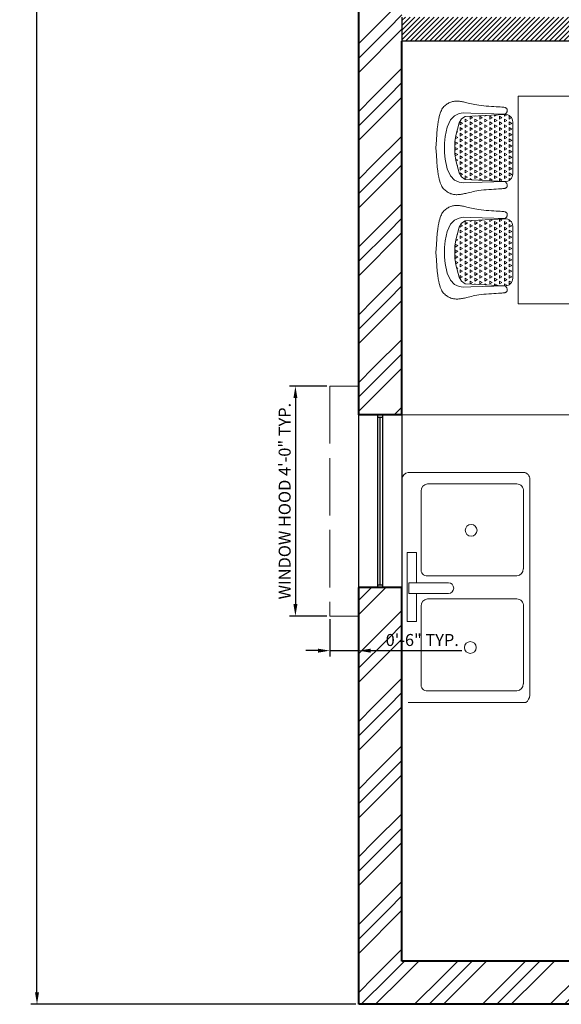
# Model space of a CAD drawing. Units: inches. Extents: x 2443635 to 2446153, y 1826255 to 1827341.
# Tile 6 of 16: x 2444253 to 2444366, y 1826861 to 1827067. Entities that reach past the tile are written whole.
import ezdxf

# ---------------------------------------------------------------- set-up
doc = ezdxf.new("R2010")
doc.units = ezdxf.units.IN
doc.linetypes.add('ACAD_ISO02W100', pattern=[15, 12, -3])
for name, color, linetype, lineweight in [('A-DIMS', 1, 'Continuous', 18), ('A-FLOR-CASE', 8, 'Continuous', 18), ('A-FLOR-FIXT', 9, 'Continuous', 18), ('A-FURN', 6, 'Continuous', 18), ('A-WALL-EXT', 7, 'Continuous', 40), ('A-WALL-INT', 9, 'Continuous', 30), ('A-WALL-OVHD', 7, 'ACAD_ISO02W100', 18), ('A-WALL-PATT', 8, 'Continuous', 13), ('A-WINDOW', 4, 'Continuous', 25)]:
    doc.layers.add(name, color=color, linetype=linetype, lineweight=lineweight)
doc.styles.get("Standard").update_dxf_attribs({"font": 'arial.ttf'})
doc.dimstyles.new('ISO-25', dxfattribs={"dimtxt": 2.5, "dimasz": 2.5, "dimexe": 1.25, "dimexo": 0.625, "dimtad": 1, "dimlunit": 4, "dimtxsty": 'Standard', "dimcen": 2.5, "dimadec": 0, "dimazin": 0, "dimtfac": 1, "dimtmove": 0, "dimatfit": 3, "dimfxl": 1, "dimarcsym": 0})

# ---------------------------------------------------------------- blocks, each defined once
blk = doc.blocks.new('*X10')
at = {"color": 0}
for p, q in [((152.44, 136.07), (152.22, 136.07)), ((152.35, 136.23), (152.44, 136.07)), ((152.62, 135.75), (152.44, 135.42)), ((152.62, 135.75), (152.81, 135.42)), ((153, 136.4), (152.81, 136.07)), ((153.19, 136.07), (152.81, 136.07)), ((153, 136.4), (153.19, 136.07)), ((153.37, 135.75), (153.19, 135.42)), ((153.37, 135.75), (153.56, 135.42)), ((153.75, 136.4), (153.56, 136.07)), ((153.94, 136.07), (153.56, 136.07)), ((153.75, 136.4), (153.94, 136.07)), ((154.12, 135.75), (153.94, 135.42)), ((154.12, 135.75), (154.31, 135.42)), ((154.5, 136.4), (154.31, 136.07)), ((154.69, 136.07), (154.31, 136.07)), ((154.5, 136.4), (154.69, 136.07)), ((154.87, 135.75), (154.69, 135.42)), ((154.87, 135.75), (155.06, 135.42)), ((155.25, 136.4), (155.06, 136.07)), ((155.44, 136.07), (155.06, 136.07)), ((155.25, 136.4), (155.44, 136.07)), ((155.62, 135.75), (155.44, 135.42)), ((155.62, 135.75), (155.81, 135.42)), ((156, 136.4), (155.81, 136.07)), ((156.19, 136.07), (155.81, 136.07)), ((156, 136.4), (156.19, 136.07)), ((156.37, 135.75), (156.19, 135.42)), ((156.37, 135.75), (156.56, 135.42)), ((156.75, 136.4), (156.56, 136.07)), ((156.94, 136.07), (156.56, 136.07)), ((156.75, 136.4), (156.94, 136.07)), ((157.12, 135.75), (156.94, 135.42)), ((157.12, 135.75), (157.31, 135.42)), ((157.5, 136.4), (157.31, 136.07)), ((157.69, 136.07), (157.31, 136.07)), ((157.5, 136.4), (157.69, 136.07)), ((157.87, 135.75), (157.69, 135.42)), ((157.87, 135.75), (158.06, 135.42)), ((158.25, 136.4), (158.06, 136.07)), ((158.44, 136.07), (158.06, 136.07)), ((158.25, 136.4), (158.44, 136.07)), ((158.62, 135.75), (158.44, 135.42)), ((158.62, 135.75), (158.81, 135.42)), ((159, 136.4), (158.81, 136.07)), ((159.19, 136.07), (158.81, 136.07)), ((159, 136.4), (159.19, 136.07)), ((159.37, 135.75), (159.19, 135.42)), ((159.37, 135.75), (159.56, 135.42)), ((159.75, 136.4), (159.56, 136.07)), ((159.94, 136.07), (159.56, 136.07)), ((159.75, 136.4), (159.94, 136.07)), ((160.12, 135.75), (159.94, 135.42)), ((160.12, 135.75), (160.31, 135.42)), ((160.48, 136.37), (160.31, 136.07)), ((160.69, 136.07), (160.31, 136.07)), ((160.54, 136.33), (160.69, 136.07)), ((160.87, 135.75), (160.69, 135.42)), ((160.87, 135.75), (160.94, 135.64)), ((152.06, 135.44), (152.06, 135.42)), ((152.06, 135.42), (152.06, 135.42)), ((152.25, 135.1), (152.09, 134.82)), ((152.44, 134.78), (152.09, 134.78)), ((152.25, 135.1), (152.44, 134.78)), ((152.81, 135.42), (152.44, 135.42)), ((152.62, 134.45), (152.44, 134.13)), ((152.62, 134.45), (152.81, 134.13)), ((153, 135.1), (152.81, 134.78)), ((153.19, 134.78), (152.81, 134.78)), ((153, 135.1), (153.19, 134.78)), ((153.56, 135.42), (153.19, 135.42)), ((153.37, 134.45), (153.19, 134.13)), ((153.37, 134.45), (153.56, 134.13)), ((153.75, 135.1), (153.56, 134.78)), ((153.94, 134.78), (153.56, 134.78)), ((153.75, 135.1), (153.94, 134.78)), ((154.31, 135.42), (153.94, 135.42)), ((154.12, 134.45), (153.94, 134.13)), ((154.12, 134.45), (154.31, 134.13)), ((154.5, 135.1), (154.31, 134.78)), ((154.69, 134.78), (154.31, 134.78)), ((154.5, 135.1), (154.69, 134.78)), ((155.06, 135.42), (154.69, 135.42)), ((154.87, 134.45), (154.69, 134.13)), ((154.87, 134.45), (155.06, 134.13)), ((155.25, 135.1), (155.06, 134.78)), ((155.44, 134.78), (155.06, 134.78)), ((155.25, 135.1), (155.44, 134.78)), ((155.81, 135.42), (155.44, 135.42)), ((155.62, 134.45), (155.44, 134.13)), ((155.62, 134.45), (155.81, 134.13)), ((156, 135.1), (155.81, 134.78)), ((156.19, 134.78), (155.81, 134.78)), ((156, 135.1), (156.19, 134.78)), ((156.56, 135.42), (156.19, 135.42)), ((156.37, 134.45), (156.19, 134.13)), ((156.37, 134.45), (156.56, 134.13)), ((156.75, 135.1), (156.56, 134.78)), ((156.94, 134.78), (156.56, 134.78)), ((156.75, 135.1), (156.94, 134.78)), ((157.31, 135.42), (156.94, 135.42)), ((157.12, 134.45), (156.94, 134.13)), ((157.12, 134.45), (157.31, 134.13)), ((157.5, 135.1), (157.31, 134.78)), ((157.69, 134.78), (157.31, 134.78)), ((157.5, 135.1), (157.69, 134.78)), ((158.06, 135.42), (157.69, 135.42)), ((157.87, 134.45), (157.69, 134.13)), ((157.87, 134.45), (158.06, 134.13)), ((158.25, 135.1), (158.06, 134.78)), ((158.44, 134.78), (158.06, 134.78)), ((158.25, 135.1), (158.44, 134.78)), ((158.81, 135.42), (158.44, 135.42)), ((158.62, 134.45), (158.44, 134.13)), ((158.62, 134.45), (158.81, 134.13)), ((159, 135.1), (158.81, 134.78)), ((159.19, 134.78), (158.81, 134.78)), ((159, 135.1), (159.19, 134.78)), ((159.56, 135.42), (159.19, 135.42)), ((159.37, 134.45), (159.19, 134.13)), ((159.37, 134.45), (159.56, 134.13)), ((159.75, 135.1), (159.56, 134.78)), ((159.94, 134.78), (159.56, 134.78)), ((159.75, 135.1), (159.94, 134.78)), ((160.31, 135.42), (159.94, 135.42)), ((160.12, 134.45), (159.94, 134.13)), ((160.12, 134.45), (160.31, 134.13)), ((160.5, 135.1), (160.31, 134.78)), ((160.69, 134.78), (160.31, 134.78)), ((160.5, 135.1), (160.69, 134.78)), ((160.94, 135.42), (160.69, 135.42)), ((160.87, 134.45), (160.69, 134.13)), ((160.87, 134.45), (160.89, 134.43)), ((152.25, 133.8), (152.15, 133.63)), ((152.44, 133.48), (152.16, 133.48)), ((152.25, 133.8), (152.44, 133.48)), ((152.81, 134.13), (152.44, 134.13)), ((152.62, 133.15), (152.44, 132.83)), ((152.62, 133.15), (152.81, 132.83)), ((153, 133.8), (152.81, 133.48)), ((153.19, 133.48), (152.81, 133.48)), ((153, 133.8), (153.19, 133.48)), ((153.56, 134.13), (153.19, 134.13)), ((153.37, 133.15), (153.19, 132.83)), ((153.37, 133.15), (153.56, 132.83)), ((153.75, 133.8), (153.56, 133.48)), ((153.94, 133.48), (153.56, 133.48)), ((153.75, 133.8), (153.94, 133.48)), ((154.31, 134.13), (153.94, 134.13)), ((154.12, 133.15), (153.94, 132.83)), ((154.12, 133.15), (154.31, 132.83)), ((154.5, 133.8), (154.31, 133.48)), ((154.69, 133.48), (154.31, 133.48)), ((154.5, 133.8), (154.69, 133.48)), ((155.06, 134.13), (154.69, 134.13)), ((154.87, 133.15), (154.69, 132.83)), ((154.87, 133.15), (155.06, 132.83)), ((155.25, 133.8), (155.06, 133.48)), ((155.44, 133.48), (155.06, 133.48)), ((155.25, 133.8), (155.44, 133.48)), ((155.81, 134.13), (155.44, 134.13)), ((155.62, 133.15), (155.44, 132.83)), ((155.62, 133.15), (155.81, 132.83)), ((156, 133.8), (155.81, 133.48)), ((156.19, 133.48), (155.81, 133.48)), ((156, 133.8), (156.19, 133.48)), ((156.56, 134.13), (156.19, 134.13)), ((156.37, 133.15), (156.19, 132.83)), ((156.37, 133.15), (156.56, 132.83)), ((156.75, 133.8), (156.56, 133.48)), ((156.94, 133.48), (156.56, 133.48)), ((156.75, 133.8), (156.94, 133.48)), ((157.31, 134.13), (156.94, 134.13)), ((157.12, 133.15), (156.94, 132.83)), ((157.12, 133.15), (157.31, 132.83)), ((157.5, 133.8), (157.31, 133.48)), ((157.69, 133.48), (157.31, 133.48)), ((157.5, 133.8), (157.69, 133.48)), ((158.06, 134.13), (157.69, 134.13)), ((157.87, 133.15), (157.69, 132.83)), ((157.87, 133.15), (158.06, 132.83)), ((158.25, 133.8), (158.06, 133.48)), ((158.44, 133.48), (158.06, 133.48)), ((158.25, 133.8), (158.44, 133.48)), ((158.81, 134.13), (158.44, 134.13)), ((158.62, 133.15), (158.44, 132.83)), ((158.62, 133.15), (158.81, 132.83)), ((159, 133.8), (158.81, 133.48)), ((159.19, 133.48), (158.81, 133.48)), ((159, 133.8), (159.19, 133.48)), ((159.56, 134.13), (159.19, 134.13)), ((159.37, 133.15), (159.19, 132.83)), ((159.37, 133.15), (159.56, 132.83)), ((159.75, 133.8), (159.56, 133.48)), ((159.94, 133.48), (159.56, 133.48)), ((159.75, 133.8), (159.94, 133.48)), ((160.31, 134.13), (159.94, 134.13)), ((160.12, 133.15), (159.94, 132.83)), ((160.12, 133.15), (160.31, 132.83)), ((160.5, 133.8), (160.31, 133.48)), ((160.69, 133.48), (160.31, 133.48)), ((160.5, 133.8), (160.69, 133.48)), ((160.87, 134.13), (160.69, 134.13)), ((160.81, 133.05), (160.69, 132.83)), ((152.25, 132.5), (152.22, 132.44)), ((152.44, 132.18), (152.23, 132.18)), ((152.25, 132.5), (152.44, 132.18)), ((152.81, 132.83), (152.44, 132.83)), ((152.62, 131.85), (152.44, 131.53)), ((152.62, 131.85), (152.81, 131.53)), ((153, 132.5), (152.81, 132.18)), ((153.19, 132.18), (152.81, 132.18)), ((153, 132.5), (153.19, 132.18)), ((153.56, 132.83), (153.19, 132.83)), ((153.37, 131.85), (153.19, 131.53)), ((153.37, 131.85), (153.56, 131.53)), ((153.75, 132.5), (153.56, 132.18)), ((153.94, 132.18), (153.56, 132.18)), ((153.75, 132.5), (153.94, 132.18)), ((154.31, 132.83), (153.94, 132.83)), ((154.12, 131.85), (153.94, 131.53)), ((154.12, 131.85), (154.31, 131.53)), ((154.5, 132.5), (154.31, 132.18)), ((154.69, 132.18), (154.31, 132.18)), ((154.5, 132.5), (154.69, 132.18)), ((155.06, 132.83), (154.69, 132.83)), ((154.87, 131.85), (154.69, 131.53)), ((154.87, 131.85), (155.06, 131.53)), ((155.25, 132.5), (155.06, 132.18)), ((155.44, 132.18), (155.06, 132.18)), ((155.25, 132.5), (155.44, 132.18)), ((155.81, 132.83), (155.44, 132.83)), ((155.62, 131.85), (155.44, 131.53)), ((155.62, 131.85), (155.81, 131.53)), ((156, 132.5), (155.81, 132.18)), ((156.19, 132.18), (155.81, 132.18)), ((156, 132.5), (156.19, 132.18)), ((156.56, 132.83), (156.19, 132.83)), ((156.37, 131.85), (156.19, 131.53)), ((156.37, 131.85), (156.56, 131.53)), ((156.75, 132.5), (156.56, 132.18)), ((156.94, 132.18), (156.56, 132.18)), ((156.75, 132.5), (156.94, 132.18)), ((157.31, 132.83), (156.94, 132.83)), ((157.12, 131.85), (156.94, 131.53)), ((157.12, 131.85), (157.31, 131.53)), ((157.5, 132.5), (157.31, 132.18)), ((157.69, 132.18), (157.31, 132.18)), ((157.5, 132.5), (157.69, 132.18)), ((158.06, 132.83), (157.69, 132.83)), ((157.87, 131.85), (157.69, 131.53)), ((157.87, 131.85), (158.06, 131.53)), ((158.25, 132.5), (158.06, 132.18)), ((158.44, 132.18), (158.06, 132.18)), ((158.25, 132.5), (158.44, 132.18)), ((158.81, 132.83), (158.44, 132.83)), ((158.62, 131.85), (158.44, 131.53)), ((158.62, 131.85), (158.81, 131.53)), ((159, 132.5), (158.81, 132.18)), ((159.19, 132.18), (158.81, 132.18)), ((159, 132.5), (159.19, 132.18)), ((159.56, 132.83), (159.19, 132.83)), ((159.37, 131.85), (159.19, 131.53)), ((159.37, 131.85), (159.56, 131.53)), ((159.75, 132.5), (159.56, 132.18)), ((159.94, 132.18), (159.56, 132.18)), ((159.75, 132.5), (159.94, 132.18)), ((160.31, 132.83), (159.94, 132.83)), ((160.12, 131.85), (159.94, 131.53)), ((160.12, 131.85), (160.31, 131.53)), ((160.5, 132.5), (160.31, 132.18)), ((160.69, 132.18), (160.31, 132.18)), ((160.5, 132.5), (160.69, 132.18)), ((160.8, 132.83), (160.69, 132.83)), ((152.29, 131.14), (152.44, 130.88)), ((152.44, 130.88), (152.3, 130.88)), ((152.81, 131.53), (152.44, 131.53)), ((152.62, 130.55), (152.44, 130.23)), ((152.62, 130.55), (152.81, 130.23)), ((153, 131.2), (152.81, 130.88)), ((153.19, 130.88), (152.81, 130.88)), ((153, 131.2), (153.19, 130.88)), ((153.56, 131.53), (153.19, 131.53)), ((153.37, 130.55), (153.19, 130.23)), ((153.37, 130.55), (153.56, 130.23)), ((153.75, 131.2), (153.56, 130.88)), ((153.94, 130.88), (153.56, 130.88)), ((153.75, 131.2), (153.94, 130.88)), ((154.31, 131.53), (153.94, 131.53)), ((154.12, 130.55), (153.94, 130.23)), ((154.12, 130.55), (154.31, 130.23)), ((154.5, 131.2), (154.31, 130.88)), ((154.69, 130.88), (154.31, 130.88)), ((154.5, 131.2), (154.69, 130.88)), ((155.06, 131.53), (154.69, 131.53)), ((154.87, 130.55), (154.69, 130.23)), ((154.87, 130.55), (155.06, 130.23)), ((155.25, 131.2), (155.06, 130.88)), ((155.44, 130.88), (155.06, 130.88)), ((155.25, 131.2), (155.44, 130.88)), ((155.81, 131.53), (155.44, 131.53)), ((155.62, 130.55), (155.44, 130.23)), ((155.62, 130.55), (155.81, 130.23)), ((156, 131.2), (155.81, 130.88)), ((156.19, 130.88), (155.81, 130.88)), ((156, 131.2), (156.19, 130.88)), ((156.56, 131.53), (156.19, 131.53)), ((156.37, 130.55), (156.19, 130.23)), ((156.37, 130.55), (156.56, 130.23)), ((156.75, 131.2), (156.56, 130.88)), ((156.94, 130.88), (156.56, 130.88)), ((156.75, 131.2), (156.94, 130.88)), ((157.31, 131.53), (156.94, 131.53)), ((157.12, 130.55), (156.94, 130.23)), ((157.12, 130.55), (157.31, 130.23)), ((157.5, 131.2), (157.31, 130.88)), ((157.69, 130.88), (157.31, 130.88)), ((157.5, 131.2), (157.69, 130.88)), ((158.06, 131.53), (157.69, 131.53)), ((157.87, 130.55), (157.69, 130.23)), ((157.87, 130.55), (158.06, 130.23)), ((158.25, 131.2), (158.06, 130.88)), ((158.44, 130.88), (158.06, 130.88)), ((158.25, 131.2), (158.44, 130.88)), ((158.81, 131.53), (158.44, 131.53)), ((158.62, 130.55), (158.44, 130.23)), ((158.62, 130.55), (158.81, 130.23)), ((159, 131.2), (158.81, 130.88)), ((159.19, 130.88), (158.81, 130.88)), ((159, 131.2), (159.19, 130.88)), ((159.56, 131.53), (159.19, 131.53)), ((159.37, 130.55), (159.19, 130.23)), ((159.37, 130.55), (159.56, 130.23)), ((159.75, 131.2), (159.56, 130.88)), ((159.94, 130.88), (159.56, 130.88)), ((159.75, 131.2), (159.94, 130.88)), ((160.31, 131.53), (159.94, 131.53)), ((160.12, 130.55), (159.94, 130.23)), ((160.12, 130.55), (160.31, 130.23)), ((160.5, 131.2), (160.31, 130.88)), ((160.69, 130.88), (160.31, 130.88)), ((160.5, 131.2), (160.69, 130.88)), ((160.74, 131.61), (160.69, 131.53)), ((160.73, 131.53), (160.69, 131.53)), ((152.81, 130.23), (152.44, 130.23)), ((153, 129.9), (152.84, 129.63)), ((153.19, 129.58), (152.93, 129.58)), ((153, 129.9), (153.19, 129.58)), ((153.56, 130.23), (153.19, 130.23)), ((153.75, 129.9), (153.56, 129.58)), ((153.94, 129.58), (153.56, 129.58)), ((153.75, 129.9), (153.94, 129.58)), ((154.31, 130.23), (153.94, 130.23)), ((154.12, 129.25), (154.09, 129.19)), ((154.12, 129.25), (154.17, 129.17)), ((154.5, 129.9), (154.31, 129.58)), ((154.69, 129.58), (154.31, 129.58)), ((154.5, 129.9), (154.69, 129.58)), ((155.06, 130.23), (154.69, 130.23)), ((154.87, 129.25), (154.74, 129.02)), ((154.87, 129.25), (155.04, 128.97)), ((155.25, 129.9), (155.06, 129.58)), ((155.44, 129.58), (155.06, 129.58)), ((155.25, 129.9), (155.44, 129.58)), ((155.81, 130.23), (155.44, 130.23)), ((155.62, 129.25), (155.44, 128.93)), ((155.62, 129.25), (155.81, 128.93)), ((156, 129.9), (155.81, 129.58)), ((156.19, 129.58), (155.81, 129.58)), ((156, 129.9), (156.19, 129.58)), ((156.56, 130.23), (156.19, 130.23)), ((156.37, 129.25), (156.19, 128.93)), ((156.37, 129.25), (156.56, 128.93)), ((156.75, 129.9), (156.56, 129.58)), ((156.94, 129.58), (156.56, 129.58)), ((156.75, 129.9), (156.94, 129.58)), ((157.31, 130.23), (156.94, 130.23)), ((157.12, 129.25), (156.94, 128.93)), ((157.12, 129.25), (157.31, 128.93)), ((157.5, 129.9), (157.31, 129.58)), ((157.69, 129.58), (157.31, 129.58)), ((157.5, 129.9), (157.69, 129.58)), ((158.06, 130.23), (157.69, 130.23)), ((157.87, 129.25), (157.69, 128.93)), ((157.87, 129.25), (158.03, 128.98)), ((158.25, 129.9), (158.06, 129.58)), ((158.44, 129.58), (158.06, 129.58)), ((158.25, 129.9), (158.44, 129.58)), ((158.81, 130.23), (158.44, 130.23)), ((158.62, 129.25), (158.53, 129.09)), ((158.62, 129.25), (158.69, 129.14)), ((159, 129.9), (158.81, 129.58)), ((159.19, 129.58), (158.81, 129.58)), ((159, 129.9), (159.19, 129.58)), ((159.56, 130.23), (159.19, 130.23)), ((159.75, 129.9), (159.56, 129.58)), ((159.94, 129.58), (159.56, 129.58)), ((159.75, 129.9), (159.94, 129.58)), ((160.31, 130.23), (159.94, 130.23)), ((155.81, 128.93), (155.44, 128.93)), ((156.56, 128.93), (156.19, 128.93)), ((157.31, 128.93), (156.94, 128.93))]:
    blk.add_line(p, q, dxfattribs=at)
blk = doc.blocks.new('A$C36D1434F')
at = {"layer": 'A-FURN'}
for p, q in [((0, 534.2), (0, 1334.2)), ((0, 1334.2), (1350, 1334.2)), ((1350, 1334.2), (1350, 534.2)), ((1350, 534.2), (0, 534.2))]:
    blk.add_line(p, q, dxfattribs=at)
for points in [[(117.6, 1418.8), (113.4, 1414.5), (109.3, 1411.1), (105.6, 1408.5), (102.1, 1406.7), (98.8, 1405.6), (95.7, 1404.9), (92.9, 1404.7), (90.4, 1404.8), (88.1, 1405.1), (85.9, 1405.5), (84, 1406.2), (82.3, 1407), (80.7, 1408), (79.3, 1409.1), (78, 1410.4), (76.9, 1411.8), (75.8, 1413.4), (74.8, 1415.4), (73.8, 1418.1), (73, 1421.7), (72.1, 1426.5), (71.4, 1432.7), (70.6, 1440.7), (69.8, 1450.6), (69.1, 1462.6), (68.3, 1476.5), (67.4, 1491.7), (66.5, 1507.9), (65.3, 1524.7), (64.1, 1541.5), (62.6, 1558.1), (60.8, 1574), (58.8, 1588.9), (56.6, 1602.7), (54.2, 1615.4), (51.7, 1627.3), (49.2, 1638.3), (46.8, 1648.5), (44.5, 1657.9), (42.3, 1666.7), (40.3, 1674.8), (38.6, 1682.4), (37.1, 1689.6), (35.8, 1696.3), (34.7, 1702.7), (33.8, 1708.8), (33.1, 1714.7), (32.5, 1720.5), (32.1, 1726.2), (31.9, 1731.8), (32, 1737.5), (32.3, 1743.1), (32.8, 1748.7), (33.7, 1754.3), (34.9, 1760), (36.5, 1765.8), (38.5, 1771.7), (40.9, 1777.6), (43.6, 1783.5), (46.7, 1789.3), (50.2, 1795.1), (54, 1800.6), (58.1, 1806), (62.6, 1811.1), (67.4, 1816), (72.6, 1820.5), (78.3, 1824.8), (84.8, 1828.9), (92, 1832.8), (100.2, 1836.5), (109.5, 1840.1), (119.9, 1843.5), (131.9, 1846.9), (146.1, 1850.2), (163.5, 1853.5), (185.3, 1856.6), (212.3, 1859.7), (245.5, 1862.7), (285.9, 1865.6), (334.5, 1868.4)], [(554.3, 1418.8), (558.6, 1414.5), (562.6, 1411.1), (566.3, 1408.5), (569.9, 1406.7), (573.1, 1405.6), (576.2, 1404.9), (579, 1404.7), (581.5, 1404.8), (583.9, 1405.1), (586, 1405.5), (587.9, 1406.2), (589.6, 1407), (591.2, 1408), (592.6, 1409.1), (593.9, 1410.4), (595.1, 1411.8), (596.2, 1413.4), (597.2, 1415.4), (598.1, 1418.1), (599, 1421.7), (599.8, 1426.5), (600.6, 1432.7), (601.3, 1440.7), (602.1, 1450.6), (602.8, 1462.6), (603.6, 1476.5), (604.5, 1491.7), (605.5, 1507.9), (606.6, 1524.7), (607.9, 1541.5), (609.4, 1558.1), (611.1, 1574), (613.1, 1588.9), (615.3, 1602.7), (617.7, 1615.4), (620.2, 1627.3), (622.7, 1638.3), (625.1, 1648.5), (627.5, 1657.9), (629.6, 1666.7), (631.6, 1674.8), (633.3, 1682.4), (634.8, 1689.6), (636.1, 1696.3), (637.2, 1702.7), (638.1, 1708.8), (638.9, 1714.7), (639.4, 1720.5), (639.8, 1726.2), (640, 1731.8), (640, 1737.5), (639.7, 1743.1), (639.1, 1748.7), (638.2, 1754.3), (637, 1760), (635.4, 1765.8), (633.4, 1771.7), (631.1, 1777.6), (628.3, 1783.5), (625.2, 1789.3), (621.7, 1795.1), (617.9, 1800.6), (613.8, 1806), (609.4, 1811.1), (604.6, 1816), (599.4, 1820.5), (593.6, 1824.8), (587.1, 1828.9), (579.9, 1832.8), (571.7, 1836.5), (562.4, 1840.1), (552, 1843.5), (540.1, 1846.9), (525.8, 1850.2), (508.2, 1853.5), (486.3, 1856.6), (458.9, 1859.7), (425.2, 1862.7), (384.1, 1865.6), (334.5, 1868.4)], [(795.7, 1418.8), (791.4, 1414.5), (787.4, 1411.1), (783.7, 1408.5), (780.1, 1406.7), (776.9, 1405.6), (773.8, 1404.9), (771, 1404.7), (768.5, 1404.8), (766.1, 1405.1), (764, 1405.5), (762.1, 1406.2), (760.4, 1407), (758.8, 1408), (757.4, 1409.1), (756.1, 1410.4), (754.9, 1411.8), (753.8, 1413.4), (752.8, 1415.4), (751.9, 1418.1), (751, 1421.7), (750.2, 1426.5), (749.4, 1432.7), (748.7, 1440.7), (747.9, 1450.6), (747.2, 1462.6), (746.4, 1476.5), (745.5, 1491.7), (744.5, 1507.9), (743.4, 1524.7), (742.1, 1541.5), (740.6, 1558.1), (738.9, 1574), (736.9, 1588.9), (734.7, 1602.7), (732.3, 1615.4), (729.8, 1627.3), (727.3, 1638.3), (724.9, 1648.5), (722.5, 1657.9), (720.4, 1666.7), (718.4, 1674.8), (716.7, 1682.4), (715.2, 1689.6), (713.9, 1696.3), (712.8, 1702.7), (711.9, 1708.8), (711.1, 1714.7), (710.6, 1720.5), (710.2, 1726.2), (710, 1731.8), (710, 1737.5), (710.3, 1743.1), (710.9, 1748.7), (711.8, 1754.3), (713, 1760), (714.6, 1765.8), (716.6, 1771.7), (718.9, 1777.6), (721.7, 1783.5), (724.8, 1789.3), (728.3, 1795.1), (732.1, 1800.6), (736.2, 1806), (740.6, 1811.1), (745.4, 1816), (750.6, 1820.5), (756.4, 1824.8), (762.9, 1828.9), (770.1, 1832.8), (778.3, 1836.5), (787.6, 1840.1), (798, 1843.5), (809.9, 1846.9), (824.2, 1850.2), (841.8, 1853.5), (863.7, 1856.6), (891.1, 1859.7), (924.8, 1862.7), (965.9, 1865.6), (1015.5, 1868.4)], [(1232.4, 1418.8), (1236.6, 1414.5), (1240.7, 1411.1), (1244.4, 1408.5), (1247.9, 1406.7), (1251.2, 1405.6), (1254.3, 1404.9), (1257.1, 1404.7), (1259.6, 1404.8), (1261.9, 1405.1), (1264.1, 1405.5), (1266, 1406.2), (1267.7, 1407), (1269.3, 1408), (1270.7, 1409.1), (1272, 1410.4), (1273.1, 1411.8), (1274.2, 1413.4), (1275.2, 1415.4), (1276.2, 1418.1), (1277, 1421.7), (1277.9, 1426.5), (1278.6, 1432.7), (1279.4, 1440.7), (1280.2, 1450.6), (1280.9, 1462.6), (1281.7, 1476.5), (1282.6, 1491.7), (1283.5, 1507.9), (1284.7, 1524.7), (1285.9, 1541.5), (1287.4, 1558.1), (1289.2, 1574), (1291.2, 1588.9), (1293.4, 1602.7), (1295.8, 1615.4), (1298.3, 1627.3), (1300.8, 1638.3), (1303.2, 1648.5), (1305.5, 1657.9), (1307.7, 1666.7), (1309.7, 1674.8), (1311.4, 1682.4), (1312.9, 1689.6), (1314.2, 1696.3), (1315.3, 1702.7), (1316.2, 1708.8), (1316.9, 1714.7), (1317.5, 1720.5), (1317.9, 1726.2), (1318.1, 1731.8), (1318, 1737.5), (1317.7, 1743.1), (1317.2, 1748.7), (1316.3, 1754.3), (1315.1, 1760), (1313.5, 1765.8), (1311.5, 1771.7), (1309.1, 1777.6), (1306.4, 1783.5), (1303.3, 1789.3), (1299.8, 1795.1), (1296, 1800.6), (1291.9, 1806), (1287.4, 1811.1), (1282.6, 1816), (1277.4, 1820.5), (1271.7, 1824.8), (1265.2, 1828.9), (1258, 1832.8), (1249.8, 1836.5), (1240.5, 1840.1), (1230.1, 1843.5), (1218.1, 1846.9), (1203.9, 1850.2), (1186.5, 1853.5), (1164.7, 1856.6), (1137.7, 1859.7), (1104.5, 1862.7), (1064.1, 1865.6), (1015.5, 1868.4)], [(117.6, 1418.8), (110.4, 1641.6), (108.9, 1691.2), (113.4, 1718.2), (127, 1748.3), (154, 1773.8), (200.6, 1794.9), (262.2, 1808.4), (304.3, 1812.9), (337.4, 1812.9)], [(554.3, 1418.8), (561.5, 1641.6), (563, 1691.2), (558.5, 1718.2), (545, 1748.3), (517.9, 1773.8), (471.3, 1794.9), (409.7, 1808.4), (367.6, 1812.9), (334.5, 1812.9)], [(795.7, 1418.8), (788.5, 1641.6), (787, 1691.2), (791.5, 1718.2), (805, 1748.3), (832.1, 1773.8), (878.7, 1794.9), (940.3, 1808.4), (982.4, 1812.9), (1015.5, 1812.9)], [(1232.4, 1418.8), (1239.6, 1641.6), (1241.1, 1691.2), (1236.6, 1718.2), (1223, 1748.3), (1196, 1773.8), (1149.4, 1794.9), (1087.8, 1808.4), (1045.7, 1812.9), (1012.6, 1812.9)], [(117.6, 449.6), (113.4, 453.9), (109.3, 457.3), (105.6, 459.9), (102.1, 461.7), (98.8, 462.8), (95.7, 463.5), (92.9, 463.7), (90.4, 463.6), (88.1, 463.3), (85.9, 462.9), (84, 462.2), (82.3, 461.4), (80.7, 460.4), (79.3, 459.3), (78, 458), (76.9, 456.6), (75.8, 455), (74.8, 453), (73.8, 450.3), (73, 446.7), (72.1, 441.9), (71.4, 435.6), (70.6, 427.7), (69.8, 417.8), (69.1, 405.8), (68.3, 391.9), (67.4, 376.7), (66.5, 360.5), (65.3, 343.7), (64.1, 326.9), (62.6, 310.3), (60.8, 294.4), (58.8, 279.5), (56.6, 265.7), (54.2, 252.9), (51.7, 241.1), (49.2, 230.1), (46.8, 219.9), (44.5, 210.5), (42.3, 201.7), (40.3, 193.6), (38.6, 186), (37.1, 178.8), (35.8, 172.1), (34.7, 165.7), (33.8, 159.6), (33.1, 153.7), (32.5, 147.9), (32.1, 142.2), (31.9, 136.6), (32, 130.9), (32.3, 125.3), (32.8, 119.7), (33.7, 114.1), (34.9, 108.4), (36.5, 102.6), (38.5, 96.7), (40.9, 90.8), (43.6, 84.9), (46.7, 79.1), (50.2, 73.3), (54, 67.8), (58.1, 62.4), (62.6, 57.3), (67.4, 52.4), (72.6, 47.9), (78.3, 43.6), (84.8, 39.5), (92, 35.6), (100.2, 31.9), (109.5, 28.3), (119.9, 24.8), (131.9, 21.5), (146.1, 18.2), (163.5, 14.9), (185.3, 11.8), (212.3, 8.7), (245.5, 5.7), (285.9, 2.8), (334.5, 0)], [(117.6, 449.6), (110.4, 226.8), (108.9, 177.2), (113.4, 150.2), (127, 120.1), (154, 94.6), (200.6, 73.5), (262.2, 60), (304.3, 55.5), (337.4, 55.5)], [(554.3, 449.6), (558.6, 453.9), (562.6, 457.3), (566.3, 459.9), (569.9, 461.7), (573.1, 462.8), (576.2, 463.5), (579, 463.7), (581.5, 463.6), (583.9, 463.3), (586, 462.9), (587.9, 462.2), (589.6, 461.4), (591.2, 460.4), (592.6, 459.3), (593.9, 458), (595.1, 456.6), (596.2, 455), (597.2, 453), (598.1, 450.3), (599, 446.7), (599.8, 441.9), (600.6, 435.6), (601.3, 427.7), (602.1, 417.8), (602.8, 405.8), (603.6, 391.9), (604.5, 376.7), (605.5, 360.5), (606.6, 343.7), (607.9, 326.9), (609.4, 310.3), (611.1, 294.4), (613.1, 279.5), (615.3, 265.7), (617.7, 252.9), (620.2, 241.1), (622.7, 230.1), (625.1, 219.9), (627.5, 210.5), (629.6, 201.7), (631.6, 193.6), (633.3, 186), (634.8, 178.8), (636.1, 172.1), (637.2, 165.7), (638.1, 159.6), (638.9, 153.7), (639.4, 147.9), (639.8, 142.2), (640, 136.6), (640, 130.9), (639.7, 125.3), (639.1, 119.7), (638.2, 114.1), (637, 108.4), (635.4, 102.6), (633.4, 96.7), (631.1, 90.8), (628.3, 84.9), (625.2, 79.1), (621.7, 73.3), (617.9, 67.8), (613.8, 62.4), (609.4, 57.3), (604.6, 52.4), (599.4, 47.9), (593.6, 43.6), (587.1, 39.5), (579.9, 35.6), (571.7, 31.9), (562.4, 28.3), (552, 24.8), (540.1, 21.5), (525.8, 18.2), (508.2, 14.9), (486.3, 11.8), (458.9, 8.7), (425.2, 5.7), (384.1, 2.8), (334.5, 0)], [(554.3, 449.6), (561.5, 226.8), (563, 177.2), (558.5, 150.2), (545, 120.1), (517.9, 94.6), (471.3, 73.5), (409.7, 60), (367.6, 55.5), (334.5, 55.5)], [(795.7, 449.6), (791.4, 453.9), (787.4, 457.3), (783.7, 459.9), (780.1, 461.7), (776.9, 462.8), (773.8, 463.5), (771, 463.7), (768.5, 463.6), (766.1, 463.3), (764, 462.9), (762.1, 462.2), (760.4, 461.4), (758.8, 460.4), (757.4, 459.3), (756.1, 458), (754.9, 456.6), (753.8, 455), (752.8, 453), (751.9, 450.3), (751, 446.7), (750.2, 441.9), (749.4, 435.6), (748.7, 427.7), (747.9, 417.8), (747.2, 405.8), (746.4, 391.9), (745.5, 376.7), (744.5, 360.5), (743.4, 343.7), (742.1, 326.9), (740.6, 310.3), (738.9, 294.4), (736.9, 279.5), (734.7, 265.7), (732.3, 252.9), (729.8, 241.1), (727.3, 230.1), (724.9, 219.9), (722.5, 210.5), (720.4, 201.7), (718.4, 193.6), (716.7, 186), (715.2, 178.8), (713.9, 172.1), (712.8, 165.7), (711.9, 159.6), (711.1, 153.7), (710.6, 147.9), (710.2, 142.2), (710, 136.6), (710, 130.9), (710.3, 125.3), (710.9, 119.7), (711.8, 114.1), (713, 108.4), (714.6, 102.6), (716.6, 96.7), (718.9, 90.8), (721.7, 84.9), (724.8, 79.1), (728.3, 73.3), (732.1, 67.8), (736.2, 62.4), (740.6, 57.3), (745.4, 52.4), (750.6, 47.9), (756.4, 43.6), (762.9, 39.5), (770.1, 35.6), (778.3, 31.9), (787.6, 28.3), (798, 24.8), (809.9, 21.5), (824.2, 18.2), (841.8, 14.9), (863.7, 11.8), (891.1, 8.7), (924.8, 5.7), (965.9, 2.8), (1015.5, 0)], [(795.7, 449.6), (788.5, 226.8), (787, 177.2), (791.5, 150.2), (805, 120.1), (832.1, 94.6), (878.7, 73.5), (940.3, 60), (982.4, 55.5), (1015.5, 55.5)], [(1232.4, 449.6), (1239.6, 226.8), (1241.1, 177.2), (1236.6, 150.2), (1223, 120.1), (1196, 94.6), (1149.4, 73.5), (1087.8, 60), (1045.7, 55.5), (1012.6, 55.5)], [(1232.4, 449.6), (1236.6, 453.9), (1240.7, 457.3), (1244.4, 459.9), (1247.9, 461.7), (1251.2, 462.8), (1254.3, 463.5), (1257.1, 463.7), (1259.6, 463.6), (1261.9, 463.3), (1264.1, 462.9), (1266, 462.2), (1267.7, 461.4), (1269.3, 460.4), (1270.7, 459.3), (1272, 458), (1273.1, 456.6), (1274.2, 455), (1275.2, 453), (1276.2, 450.3), (1277, 446.7), (1277.9, 441.9), (1278.6, 435.6), (1279.4, 427.7), (1280.2, 417.8), (1280.9, 405.8), (1281.7, 391.9), (1282.6, 376.7), (1283.5, 360.5), (1284.7, 343.7), (1285.9, 326.9), (1287.4, 310.3), (1289.2, 294.4), (1291.2, 279.5), (1293.4, 265.7), (1295.8, 252.9), (1298.3, 241.1), (1300.8, 230.1), (1303.2, 219.9), (1305.5, 210.5), (1307.7, 201.7), (1309.7, 193.6), (1311.4, 186), (1312.9, 178.8), (1314.2, 172.1), (1315.3, 165.7), (1316.2, 159.6), (1316.9, 153.7), (1317.5, 147.9), (1317.9, 142.2), (1318.1, 136.6), (1318, 130.9), (1317.7, 125.3), (1317.2, 119.7), (1316.3, 114.1), (1315.1, 108.4), (1313.5, 102.6), (1311.5, 96.7), (1309.1, 90.8), (1306.4, 84.9), (1303.3, 79.1), (1299.8, 73.3), (1296, 67.8), (1291.9, 62.4), (1287.4, 57.3), (1282.6, 52.4), (1277.4, 47.9), (1271.7, 43.6), (1265.2, 39.5), (1258, 35.6), (1249.8, 31.9), (1240.5, 28.3), (1230.1, 24.8), (1218.1, 21.5), (1203.9, 18.2), (1186.5, 14.9), (1164.7, 11.8), (1137.7, 8.7), (1104.5, 5.7), (1064.1, 2.8), (1015.5, 0)]]:
    blk.add_lwpolyline(points, dxfattribs=at)
for points in [[(337.5, 1745.3), (375.1, 1745.3), (417.2, 1739.3), (498.4, 1718.2), (523.9, 1703.2), (540.5, 1679.2), (554.2, 1421.5, -0.429937), (505.2, 1369.7), (166.8, 1369.7, -0.429937), (117.8, 1421.5), (131.6, 1679.2), (148.1, 1703.2), (173.7, 1718.2), (254.8, 1739.3), (296.9, 1745.3), (334.5, 1745.3)], [(1012.5, 1745.3), (974.9, 1745.3), (932.8, 1739.3), (851.6, 1718.2), (826.1, 1703.2), (809.5, 1679.2), (795.8, 1421.5, 0.429937), (844.8, 1369.7), (1183.2, 1369.7, 0.429937), (1232.2, 1421.5), (1218.4, 1679.2), (1201.9, 1703.2), (1176.3, 1718.2), (1095.2, 1739.3), (1053.1, 1745.3), (1015.5, 1745.3)], [(337.5, 123.1), (375.1, 123.1), (417.2, 129.1), (498.4, 150.2), (523.9, 165.2), (540.5, 189.2), (554.2, 446.9, 0.429937), (505.2, 498.7), (166.8, 498.7, 0.429937), (117.8, 446.9), (131.6, 189.2), (148.1, 165.2), (173.7, 150.2), (254.8, 129.1), (296.9, 123.1), (334.5, 123.1)], [(1012.5, 123.1), (974.9, 123.1), (932.8, 129.1), (851.6, 150.2), (826.1, 165.2), (809.5, 189.2), (795.8, 446.9, -0.429937), (844.8, 498.7), (1183.2, 498.7, -0.429937), (1232.2, 446.9), (1218.4, 189.2), (1201.9, 165.2), (1176.3, 150.2), (1095.2, 129.1), (1053.1, 123.1), (1015.5, 123.1)]]:
    blk.add_lwpolyline(points, format="xyb", dxfattribs=at)
at = {"layer": 'A-FURN', "xscale": 49.09090909079987, "yscale": 49.09090909079987, "zscale": 49.09090909079987, "rotation": 180}
blk.add_blockref('*X10', (8018.7, 8071.8), dxfattribs=at)
at = {"layer": 'A-FURN', "extrusion": (0, 0, -1), "xscale": 49.09090909079987, "yscale": 49.09090909079987, "zscale": -49.09090909079999, "rotation": 180}
blk.add_blockref('*X10', (6668.7, 8071.8), dxfattribs=at)
at = {"layer": 'A-FURN', "extrusion": (0, 0, -1), "xscale": 49.09090909079987, "yscale": 49.09090909079987, "zscale": -49.09090909079999}
blk.add_blockref('*X10', (-8018.7, -6203.4), dxfattribs=at)
at = {"layer": 'A-FURN', "xscale": 49.09090909079987, "yscale": 49.09090909079987, "zscale": 49.09090909079987}
blk.add_blockref('*X10', (-6668.7, -6203.4), dxfattribs=at)
blk = doc.blocks.new('BASE-CABINET-L-PLAN')
at = {"transparency": 33554687}
for p, q in [((0, 78), (36, 78)), ((36, 0), (36, 78)), ((120, 0), (36, 0))]:
    blk.add_line(p, q, dxfattribs=at)
blk = doc.blocks.new('WIN-36-PLAN')
at = {"transparency": 33554687}
for p, q in [((0, 9), (36, 9)), ((0, 0), (0, 9)), ((36, 9), (36, 0)), ((0, 5), (36, 5)), ((0.5, 4), (0.5, 5)), ((0.5, 4.5), (35.5, 4.5)), ((35.5, 5), (35.5, 4)), ((0, 4), (36, 4)), ((36, 0), (0, 0))]:
    blk.add_line(p, q, dxfattribs=at)
blk = doc.blocks.new('WINDOW-HOOD-48-PLAN')
at = {"transparency": 33554687}
for p, q in [((0, 6), (0, 0)), ((48, 0), (48, 6)), ((0, 0), (48, 0))]:
    blk.add_line(p, q, dxfattribs=at)
blk = doc.blocks.new('*D60')
at = {"layer": 'A-DIMS', "color": 0, "lineweight": -2, "transparency": 16777216}
for p, q in [((2444316.93, 1826990.29), (2444309.1, 1826990.29)), ((2444310.35, 1826987.79), (2444310.35, 1826944.79)), ((2444316.93, 1826942.29), (2444309.1, 1826942.29))]:
    blk.add_line(p, q, dxfattribs=at)
at = {"layer": 'A-DIMS', "color": 0, "transparency": 16777216}
for points in [[(2444309.94, 1826987.79), (2444310.77, 1826987.79), (2444310.35, 1826990.29)], [(2444309.94, 1826944.79), (2444310.77, 1826944.79), (2444310.35, 1826942.29)]]:
    blk.add_solid(points, dxfattribs=at)
at = {"layer": 'Defpoints', "color": 0, "transparency": 16777216}
for p in [(2444317.55, 1826990.29), (2444310.35, 1826942.29), (2444317.55, 1826942.29)]:
    blk.add_point(p, dxfattribs=at)
at = {"layer": 'A-DIMS', "color": 0, "transparency": 16777216, "insert": (2444308.43, 1826966.29), "char_height": 2.5, "attachment_point": 5, "rotation": 90}
blk.add_mtext('WINDOW HOOD 4\'-0" TYP.', dxfattribs=at)
blk = doc.blocks.new('*D61')
at = {"layer": 'A-DIMS', "color": 0, "lineweight": -2, "transparency": 16777216}
for p, q in [((2444317.55, 1826941.66), (2444317.55, 1826933.84)), ((2444323.55, 1826941.66), (2444323.55, 1826933.84)), ((2444315.05, 1826935.09), (2444312.55, 1826935.09)), ((2444317.55, 1826935.09), (2444323.55, 1826935.09)), ((2444326.05, 1826935.09), (2444345.04, 1826935.09))]:
    blk.add_line(p, q, dxfattribs=at)
at = {"layer": 'A-DIMS', "color": 0, "transparency": 16777216}
for points in [[(2444315.05, 1826935.5), (2444315.05, 1826934.67), (2444317.55, 1826935.09)], [(2444326.05, 1826935.5), (2444326.05, 1826934.67), (2444323.55, 1826935.09)]]:
    blk.add_solid(points, dxfattribs=at)
at = {"layer": 'Defpoints', "color": 0, "transparency": 16777216}
for p in [(2444317.55, 1826942.29), (2444323.55, 1826942.29), (2444323.55, 1826935.09)]:
    blk.add_point(p, dxfattribs=at)
at = {"layer": 'A-DIMS', "color": 0, "transparency": 16777216, "insert": (2444336.8, 1826936.99), "char_height": 2.5, "attachment_point": 5}
blk.add_mtext('0\'-6" TYP.', dxfattribs=at)
blk = doc.blocks.new('*D95')
at = {"layer": 'A-DIMS', "color": 0, "lineweight": -2, "transparency": 16777216}
for p, q in [((2444322.93, 1827305.29), (2444255.2, 1827305.29)), ((2444256.45, 1826863.79), (2444256.45, 1827302.79)), ((2444322.93, 1826861.29), (2444255.2, 1826861.29))]:
    blk.add_line(p, q, dxfattribs=at)
at = {"layer": 'A-DIMS', "color": 0, "transparency": 16777216}
for points in [[(2444256.04, 1827302.79), (2444256.87, 1827302.79), (2444256.45, 1827305.29)], [(2444256.04, 1826863.79), (2444256.87, 1826863.79), (2444256.45, 1826861.29)]]:
    blk.add_solid(points, dxfattribs=at)
at = {"layer": 'Defpoints', "color": 0, "transparency": 16777216}
for p in [(2444256.45, 1827305.29), (2444323.55, 1827305.29), (2444323.55, 1826861.29)]:
    blk.add_point(p, dxfattribs=at)
at = {"layer": 'A-DIMS', "color": 0, "transparency": 16777216, "insert": (2444254.55, 1827083.29), "char_height": 2.5, "attachment_point": 5, "rotation": 90}
blk.add_mtext('37\'-0"', dxfattribs=at)

msp = doc.modelspace()

# ---------------------------------------------------------------- hatches: boundary and pattern name
at = {"layer": 'A-WALL-PATT'}
h = msp.add_hatch(dxfattribs=at)
h.set_pattern_fill('GOST_GROUND', color=256)
h.paths.add_polyline_path([(2444332.553, 1827147.288), (2444332.553, 1827152.288), (2444332.553, 1827161.288), (2444328.953, 1827161.288), (2444323.553, 1827161.288), (2444323.553, 1826984.288), (2444332.553, 1826984.288), (2444332.553, 1827062.288), (2444332.553, 1827067.288)])
h.paths.add_polyline_path([(2444332.553, 1826948.288), (2444323.553, 1826948.288), (2444323.553, 1826861.288), (2444374.553, 1826861.288), (2444374.553, 1826870.288), (2444332.553, 1826870.288)])
h.paths.add_polyline_path([(2444647.553, 1826941.288), (2444638.553, 1826941.288), (2444638.553, 1826935.288), (2444638.553, 1826930.288), (2444638.553, 1826870.288), (2444457.553, 1826870.288), (2444452.553, 1826870.288), (2444410.553, 1826870.288), (2444410.553, 1826861.288), (2444647.553, 1826861.288)])
h.paths.add_polyline_path([(2444647.553, 1827161.288), (2444638.553, 1827161.288), (2444638.553, 1827152.288), (2444638.553, 1827147.288), (2444638.553, 1826989.288), (2444647.553, 1826989.288)])
h.paths.add_polyline_path([(2444647.553, 1827305.288), (2444494.553, 1827305.288), (2444494.553, 1827296.288), (2444498.051, 1827296.288), (2444638.553, 1827296.288), (2444638.553, 1827254.288), (2444647.553, 1827254.288)])
h.paths.add_polyline_path([(2444476.553, 1827305.288), (2444323.553, 1827305.288), (2444323.553, 1827254.288), (2444332.553, 1827254.288), (2444332.553, 1827296.288), (2444346.141, 1827296.288), (2444476.553, 1827296.288)])
h.paths.add_polyline_path([(2444323.553, 1827305.288), (2444282.553, 1827305.288), (2444282.553, 1827147.459), (2444323.553, 1827147.459), (2444323.553, 1827152.459), (2444287.553, 1827152.459), (2444287.553, 1827300.288), (2444323.553, 1827300.288)])
h.paths.add_polyline_path([(2444688.553, 1827305.288), (2444647.553, 1827305.288), (2444647.553, 1827300.288), (2444683.553, 1827300.288), (2444683.553, 1827152.362), (2444647.553, 1827152.362), (2444647.553, 1827147.362), (2444688.553, 1827147.362)])
h = msp.add_hatch(dxfattribs=at)
h.set_pattern_fill('JIS_WOOD', color=256)
h.paths.add_polyline_path([(2444481.553, 1827095.288), (2444476.553, 1827095.288), (2444476.553, 1827067.288), (2444332.553, 1827067.288), (2444332.553, 1827062.288), (2444481.553, 1827062.288)])
h.paths.add_polyline_path([(2444457.553, 1827020.288), (2444452.553, 1827020.288), (2444452.553, 1826870.288), (2444457.553, 1826870.288), (2444457.553, 1826930.288), (2444530.053, 1826930.288), (2444530.053, 1826935.288), (2444457.553, 1826935.288)])
h.paths.add_polyline_path([(2444457.553, 1827062.288), (2444452.553, 1827062.288), (2444452.553, 1827056.288), (2444457.553, 1827056.288)])
h.paths.add_polyline_path([(2444638.553, 1826935.288), (2444566.053, 1826935.288), (2444566.053, 1826930.288), (2444638.553, 1826930.288)])
h.paths.add_polyline_path([(2444638.553, 1827152.288), (2444518.553, 1827152.288), (2444518.553, 1827156.288), (2444513.553, 1827156.288), (2444513.553, 1827147.288), (2444638.553, 1827147.288)])
h.paths.add_polyline_path([(2444518.553, 1827296.288), (2444513.553, 1827296.288), (2444513.553, 1827224.288), (2444507.553, 1827224.288), (2444507.553, 1827223.788), (2444507.553, 1827219.288), (2444513.553, 1827219.288), (2444513.553, 1827192.288), (2444518.553, 1827192.288)])
h.paths.add_polyline_path([(2444477.553, 1827223.788, -0.0041669), (2444477.557, 1827224.288), (2444457.553, 1827224.288), (2444457.553, 1827296.288), (2444452.553, 1827296.288), (2444452.553, 1827192.288), (2444457.553, 1827192.288), (2444457.553, 1827219.288), (2444477.553, 1827219.288)])
h.paths.add_polyline_path([(2444481.553, 1827152.288), (2444332.553, 1827152.288), (2444332.553, 1827147.288), (2444476.553, 1827147.288), (2444476.553, 1827137.288), (2444481.553, 1827137.288)])

# ---------------------------------------------------------------- linework, layer by layer
at = {"layer": 'A-FLOR-FIXT'}
for p, q in [((2444332.553, 1826925.788), (2444332.553, 1826970.788)), ((2444333.886, 1826972.279), (2444357.886, 1826972.279)), ((2444359.219, 1826970.779), (2444359.219, 1826925.788)), ((2444337.886, 1826969.879), (2444356.553, 1826969.879)), ((2444336.553, 1826952.179), (2444336.553, 1826968.379)), ((2444357.886, 1826968.379), (2444357.886, 1826952.179)), ((2444333.637, 1826955.55), (2444333.637, 1826941.15)), ((2444335.636, 1826955.55), (2444333.637, 1826955.55)), ((2444335.636, 1826949.262), (2444335.636, 1826955.55)), ((2444356.553, 1826950.679), (2444337.886, 1826950.679)), ((2444342.253, 1826949.262), (2444333.982, 1826949.262)), ((2444333.982, 1826949.262), (2444333.982, 1826947.027)), ((2444333.982, 1826947.027), (2444342.253, 1826947.027)), ((2444335.636, 1826941.15), (2444335.636, 1826947.027)), ((2444336.553, 1826928.179), (2444336.553, 1826944.379)), ((2444337.886, 1826945.879), (2444356.553, 1826945.879)), ((2444357.886, 1826944.379), (2444357.886, 1826928.179)), ((2444333.637, 1826941.15), (2444335.636, 1826941.15)), ((2444356.553, 1826926.679), (2444337.886, 1826926.679)), ((2444358.386, 1826924.288), (2444333.886, 1826924.279))]:
    msp.add_line(p, q, dxfattribs=at)
for centre in [(2444346.997, 1826960.197), (2444346.829, 1826935.745)]:
    msp.add_circle(centre, 1.233, dxfattribs=at)
for centre, radius, start, end in [((2444334.053, 1826970.788), 1.501, 96.40919, 180.00001), ((2444357.886, 1826970.937), 1.343, 353.26708, 89.99999), ((2444338.063, 1826968.379), 1.51, 96.73295, 179.99997), ((2444356.553, 1826968.537), 1.343, 353.26708, 89.99999), ((2444337.886, 1826952.022), 1.343, 173.26708, 269.99999), ((2444356.375, 1826952.179), 1.51, 276.73295, 359.99997), ((2444342.253, 1826948.145), 1.117, 270, 90), ((2444338.063, 1826944.379), 1.51, 96.73295, 179.99997), ((2444356.553, 1826944.537), 1.343, 353.26708, 89.99999), ((2444337.886, 1826928.022), 1.343, 173.26708, 269.99999), ((2444356.375, 1826928.179), 1.51, 276.73295, 359.99997), ((2444357.453, 1826925.788), 1.767, 301.89079, 360)]:
    msp.add_arc(centre, radius, start, end, dxfattribs=at)
at = {"layer": 'A-WALL-EXT'}
for p, q in [((2444323.553, 1826984.288), (2444323.553, 1827162.338)), ((2444332.553, 1826984.288), (2444332.553, 1827062.288)), ((2444332.553, 1826984.288), (2444323.553, 1826984.288)), ((2444323.553, 1826861.288), (2444323.553, 1826948.288)), ((2444332.553, 1826948.288), (2444323.553, 1826948.288)), ((2444332.553, 1826870.288), (2444332.553, 1826948.288)), ((2444374.553, 1826870.288), (2444332.553, 1826870.288)), ((2444374.553, 1826861.288), (2444323.553, 1826861.288))]:
    msp.add_line(p, q, dxfattribs=at)
at = {"layer": 'A-WALL-INT'}
for p in [(2444332.553, 1827067.288), (2444481.553, 1827062.288)]:
    msp.add_line(p, (2444332.553, 1827062.288), dxfattribs=at)
at = {"layer": 'A-WINDOW'}
for p, q in [((2444323.553, 1826984.288), (2444332.553, 1826984.288)), ((2444332.553, 1826948.288), (2444323.553, 1826948.288))]:
    msp.add_line(p, q, dxfattribs=at)

# ---------------------------------------------------------------- block references
at = {"layer": 'A-FLOR-CASE', "transparency": 33554687}
msp.add_blockref('BASE-CABINET-L-PLAN', (2444332.553, 1826906.288), dxfattribs=at)
at = {"layer": 'A-FURN', "xscale": 0.032113081480791, "yscale": 0.032113081480791, "zscale": 0.032113081480791, "rotation": 270}
msp.add_blockref('A$C36D1434F', (2444339.652, 1827050.79), dxfattribs=at)
at = {"layer": 'A-WALL-OVHD', "transparency": 33554687, "rotation": 270.0000000010816}
msp.add_blockref('WINDOW-HOOD-48-PLAN', (2444317.553, 1826990.288), dxfattribs=at)
at = {"layer": 'A-WINDOW', "transparency": 33554687, "rotation": 90.00000000244133}
msp.add_blockref('WIN-36-PLAN', (2444332.553, 1826948.288), dxfattribs=at)

# ---------------------------------------------------------------- dimensions: what is measured, and where the dimension line sits
at = {"layer": 'A-DIMS', "transparency": 33554687}
dim = msp.add_linear_dim(base=(2444256.453, 1827305.288), p1=(2444323.553, 1826861.288), p2=(2444323.553, 1827305.288), angle=90, dimstyle='ISO-25', override={"dimdec": 1, "dimlfac": 1, "dimrnd": 0, "dimzin": 1, "dimdsep": 46, "dimlunit": 4, "dimfrac": 2}, dxfattribs=at)
dim.commit()
dim.dimension.update_dxf_attribs({"geometry": '*D95', "text_midpoint": (2444254.55, 1827083.288)})
dim = msp.add_linear_dim(base=(2444310.353, 1826942.288), p1=(2444317.553, 1826990.288), p2=(2444317.553, 1826942.288), angle=270, text='WINDOW HOOD <> TYP.', dimstyle='ISO-25', override={"dimdec": 1, "dimlfac": 1, "dimrnd": 0, "dimzin": 1, "dimdsep": 46, "dimlunit": 4, "dimfrac": 2}, dxfattribs=at)
dim.commit()
dim.dimension.update_dxf_attribs({"geometry": '*D60', "text_midpoint": (2444308.434, 1826966.288)})
dim = msp.add_linear_dim(base=(2444323.553, 1826935.088), p1=(2444317.553, 1826942.288), p2=(2444323.553, 1826942.288), text='<> TYP.', dimstyle='ISO-25', override={"dimdec": 1, "dimlfac": 1, "dimrnd": 0, "dimzin": 1, "dimdsep": 46, "dimlunit": 4, "dimfrac": 2}, dxfattribs=at)
dim.commit()
dim.dimension.update_dxf_attribs({"geometry": '*D61', "text_midpoint": (2444336.797, 1826936.989)})

doc.saveas('drawing.dxf')
